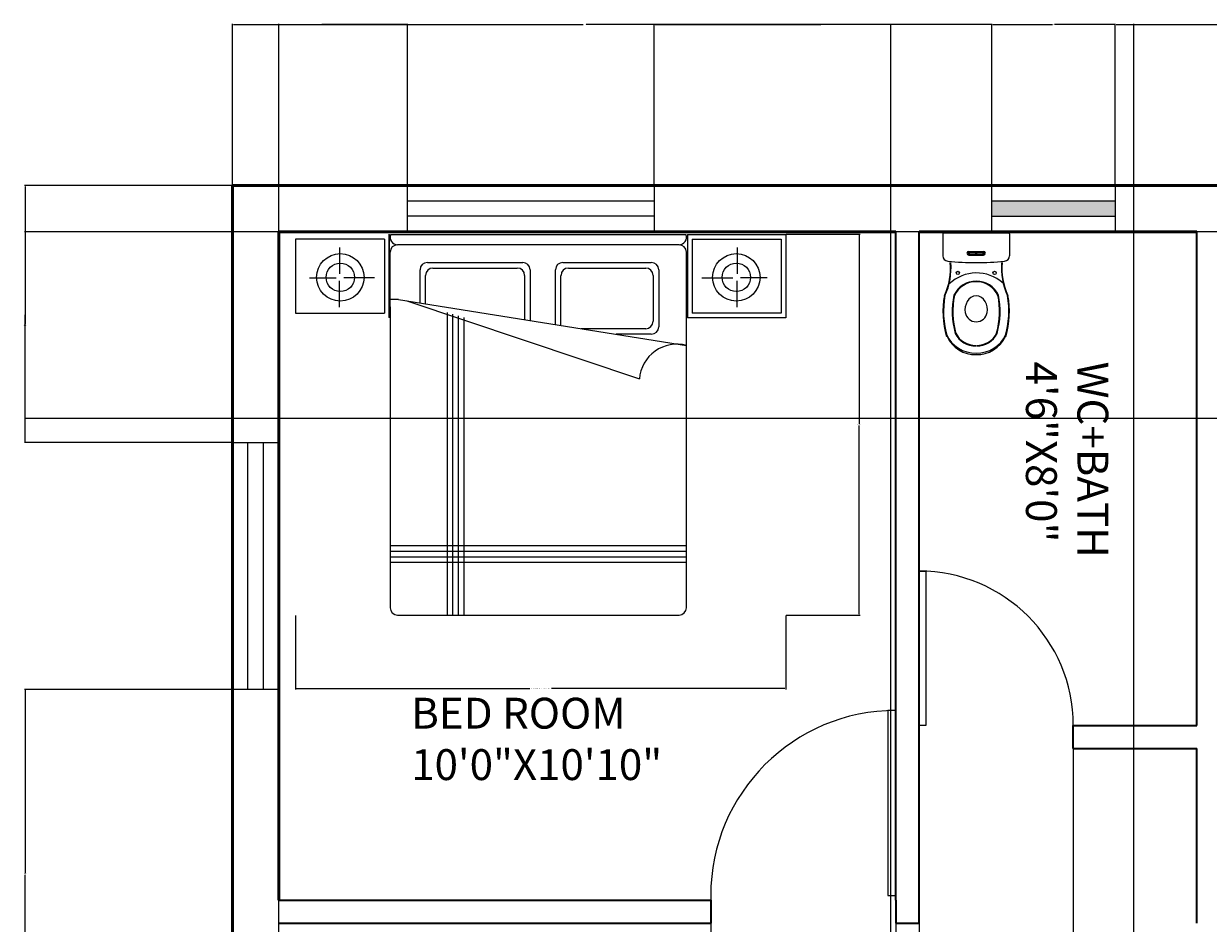
# Model space of a CAD drawing. Units: feet. Extents: x 2664 to 3060, y 1318 to 2005.
# Tile 4 of 5: x 2664 to 2894, y 1830 to 2005. Entities that reach past the tile are written whole.
import ezdxf

# ---------------------------------------------------------------- set-up
doc = ezdxf.new("R2010")
doc.units = ezdxf.units.FT
for name, color, linetype, lineweight in [('A-ANNO-DIMS', 2, 'Continuous', 18), ('A-AREA-IDEN', 109, 'Continuous', 18), ('A-WALL-EXTR', 130, 'Continuous', 50), ('DOOR', 249, 'Continuous', 25), ('FURNITURE', 240, 'Continuous', 13), ('SANITARY', 50, 'Continuous', 13)]:
    doc.layers.add(name, color=color, linetype=linetype, lineweight=lineweight)
for name, color, linetype, lineweight, true_color in [('A-GLAZ', 222, 'Continuous', 18, 0xd4008b), ('A-VENT-PATT', 219, 'Continuous', 13, 0x642165), ('A-WALL-INTR', 41, 'Continuous', 35, 0xf5dd7a), ('VENT', 95, 'Continuous', 18, 0x46b72a)]:
    doc.layers.add(name, color=color, linetype=linetype, lineweight=lineweight, true_color=true_color)
doc.styles.get("Standard").update_dxf_attribs({"font": 'arial.ttf'})
doc.dimstyles.get("Standard").update_dxf_attribs({"dimtxt": 0.18, "dimasz": 0.18, "dimexe": 0.18, "dimexo": 0.0625, "dimgap": 0.09, "dimtad": 0, "dimtih": 1, "dimtoh": 1, "dimdec": 4, "dimzin": 0, "dimdsep": 46, "dimtxsty": 'Standard', "dimcen": 0.09, "dimadec": 0, "dimazin": 0, "dimtfac": 1, "dimtdec": 4, "dimtofl": 0, "dimtmove": 0, "dimatfit": 3, "dimfxl": 1, "dimtolj": 1, "dimtzin": 0, "dimarcsym": 0})

# ---------------------------------------------------------------- blocks, each defined once
blk = doc.blocks.new('*U3')
for p, q in [((0, 0), (0, -6)), ((-40, 0), (-40, -6))]:
    blk.add_line(p, q)
blk.add_lwpolyline([(0, 0), (0, 40), (-1.75, 40), (-1.75, 0)], close=True)
blk.add_arc((0, 0), 40, 90, 180)
blk = doc.blocks.new('*U2')
for p, q in [((0, 0), (0, -6)), ((40, 0), (40, -6))]:
    blk.add_line(p, q)
blk.add_lwpolyline([(0, 0), (0, 40), (1.75, 40), (1.75, 0)], close=True)
blk.add_arc((0, 0), 40, 0, 90)
blk = doc.blocks.new('BED-DOUBLE-WITH-NIGHTSTANDS')
for p, q in [((-29.54, 0), (-29.54, -16.21)), ((-30.37, -0.95), (-47.65, -0.95)), ((-47.65, -0.95), (-47.65, -15.35)), ((-30.37, -0.95), (-30.37, -15.35)), ((-29.47, -0.05), (-29.47, -16.25)), ((28.27, -0.11), (-29.17, -0.11)), ((26.92, -2.06), (-27.82, -2.06)), ((28.57, -0.05), (47.65, -0.05)), ((28.57, -0.05), (28.57, -16.25)), ((29.47, -0.95), (46.75, -0.95)), ((29.47, -0.95), (29.47, -15.35)), ((46.75, -0.95), (46.75, -15.35)), ((47.65, -0.05), (47.65, -16.25)), ((-39.11, -2.58), (-39.11, -7.74)), ((-29.26, -14.16), (-29.26, -3.5)), ((28.36, -72.65), (28.36, -3.5)), ((38.21, -2.58), (38.21, -7.74)), ((-22.01, -5.5), (-3.48, -5.5)), ((-20.93, -6.58), (-4.56, -6.58)), ((4.33, -5.5), (21.52, -5.5)), ((5.41, -6.58), (20.44, -6.58)), ((-44.95, -8.46), (-39.75, -8.46)), ((-39.11, -14.22), (-39.11, -9.06)), ((-32.27, -8.46), (-38.27, -8.46)), ((-23.45, -13.32), (-23.45, -6.94)), ((-22.37, -13.47), (-22.37, -8.02)), ((-3.12, -8.02), (-3.12, -16.63)), ((-2.04, -6.94), (-2.04, -16.8)), ((2.88, -17.58), (2.88, -6.94)), ((3.96, -17.76), (3.96, -8.02)), ((21.88, -8.02), (21.88, -16.94)), ((22.96, -6.94), (22.96, -18.02)), ((31.37, -8.46), (37.37, -8.46)), ((38.21, -14.22), (38.21, -9.06)), ((44.05, -8.46), (38.85, -8.46)), ((-27.62, -12.73), (-29.26, -12.73)), ((-27.62, -12.73), (28.36, -21.64)), ((-26, -12.96), (19.2, -28.15)), ((-47.65, -15.35), (-30.37, -15.35)), ((-29.26, -14.16), (-29.26, -72.65)), ((-18.14, -74.09), (-18.14, -15.24)), ((-17.06, -74.09), (-17.06, -15.55)), ((-15.97, -74.09), (-15.97, -15.86)), ((46.75, -15.35), (29.47, -15.35)), ((-14.89, -74.09), (-14.89, -16.18)), ((20.44, -18.38), (7.87, -18.38)), ((47.65, -16.25), (28.57, -16.25)), ((21.52, -19.46), (14.66, -19.46)), ((28.36, -60.64), (-29.26, -60.64)), ((28.36, -61.72), (-29.26, -61.72)), ((28.36, -62.8), (-29.26, -62.8)), ((28.36, -63.88), (-29.26, -63.88)), ((-27.82, -74.09), (26.92, -74.09))]:
    blk.add_line(p, q)
for centre, radius in [((-38.95, -8.4), 4.61), ((38.05, -8.4), 4.61), ((-38.95, -8.4), 2.77), ((38.05, -8.4), 2.77)]:
    blk.add_circle(centre, radius)
for centre, radius, start, end in [((-27.82, -0.62), 1.44, 159.2884, 270), ((-27.82, -3.5), 1.44, 90, 180), ((26.92, -0.62), 1.44, 270, 20.7116), ((26.92, -3.5), 1.44, 0, 90), ((-22.01, -6.94), 1.44, 90, 180), ((-20.93, -8.02), 1.44, 90, 180), ((-4.56, -8.02), 1.44, 0, 90), ((-3.48, -6.94), 1.44, 0, 90), ((4.33, -6.94), 1.44, 90, 180), ((5.41, -8.02), 1.44, 90, 180), ((20.44, -8.02), 1.44, 0, 90), ((21.52, -6.94), 1.44, 0, 90), ((20.44, -16.94), 1.44, 270, 0), ((21.52, -18.02), 1.44, 270, 0), ((26.5, -28.71), 7.32, 75.237, 175.5647), ((-27.82, -72.65), 1.44, 180, 270), ((26.92, -72.65), 1.44, 270, 0)]:
    blk.add_arc(centre, radius, start, end)
blk = doc.blocks.new('WC-FLOOR-MOUNT')
for p, q in [((-6.3, 0), (6.3, 0)), ((-6.48, -0.18), (-6.48, -4.43)), ((6.48, -0.18), (6.48, -4.43)), ((-1.44, -3.6), (1.44, -3.6)), ((-1.44, -3.71), (1.44, -3.71)), ((-1.44, -3.82), (-0.18, -3.82)), ((-1.44, -4.11), (-0.18, -4.11)), ((-1.44, -4.21), (1.44, -4.21)), ((-1.44, -4.32), (1.44, -4.32)), ((-0.07, -3.93), (-0.07, -4)), ((0.07, -3.93), (0.07, -4)), ((0.18, -3.82), (1.44, -3.82)), ((0.18, -4.11), (1.44, -4.11))]:
    blk.add_line(p, q)
for centre, radius in [((-1.42, -3.96), 0.112), ((-1.42, -3.96), 0.0402), ((1.42, -3.96), 0.112), ((1.42, -3.96), 0.0402), ((-3.57, -7.78), 0.318), ((3.57, -7.78), 0.318)]:
    blk.add_circle(centre, radius)
for centre, radius, start, end in [((-6.3, -0.18), 0.18, 90, 180), ((6.3, -0.18), 0.18, 0, 90), ((-5.4, -4.43), 1.08, 180, 264.6037), ((-1.44, -3.96), 0.36, 90, 180), ((-1.44, -3.96), 0.36, 180, 270), ((-1.44, -3.96), 0.252, 90, 180), ((-1.44, -3.96), 0.252, 180, 270), ((-1.44, -3.96), 0.144, 90, 270), ((-0.18, -3.93), 0.108, 0, 90), ((-0.18, -4), 0.108, 270, 0), ((0.18, -3.93), 0.108, 90, 180), ((0.18, -4), 0.108, 180, 270), ((1.44, -3.96), 0.36, 0, 90), ((1.44, -3.96), 0.252, 0, 90), ((1.44, -3.96), 0.144, 270, 90), ((1.44, -3.96), 0.36, 270, 0), ((1.44, -3.96), 0.252, 270, 0), ((5.4, -4.43), 1.08, 275.3963, 0), ((-17.58, -6.84), 12.59, 334.9634, 4.9109), ((-17.58, -6.84), 12.69, 334.9634, 4.9109), ((0, 52.77), 58.53, 264.6037, 275.3963), ((17.58, -6.84), 12.69, 175.0891, 205.0366), ((17.58, -6.84), 12.59, 175.0891, 205.0366), ((0.06, -15.51), 7.72, 48.0834, 133.5369), ((0, -14.17), 4.8, 25.6263, 154.3737), ((0, -14.17), 4.69, 25.6263, 154.3737), ((11.03, -15.28), 17.49, 169.7326, 196.2187), ((11.03, -15.28), 17.38, 169.7326, 196.2187), ((11.03, -15.28), 15.69, 168.2525, 195.7257), ((11.03, -15.28), 15.58, 168.2525, 196.2187), ((1.08, -14.97), 3.26, 149.7876, 189.0746), ((0, -14.17), 1.92, 25.6263, 154.3737), ((-1.08, -14.97), 3.26, 350.9254, 30.2124), ((-11.03, -15.28), 15.58, 344.3098, 11.7475), ((-11.03, -15.28), 15.69, 344.2743, 11.7475), ((-11.03, -15.28), 17.38, 343.7813, 10.2674), ((-11.03, -15.28), 17.49, 343.7813, 10.2674), ((0, -15.12), 2.16, 189.6495, 350.3505), ((-0.18, -17.24), 6.13, 204.3045, 271.6847), ((-0.18, -17.65), 6.02, 204.3045, 271.6847), ((-0.18, -17.65), 4.32, 205.8912, 271.6847), ((-0.18, -17.65), 4.22, 206.0212, 271.6847), ((0.18, -17.24), 6.13, 268.3153, 335.6955), ((0.18, -17.65), 6.02, 268.3153, 335.6955), ((0.18, -17.65), 4.32, 268.3153, 334.1088), ((0.18, -17.65), 4.22, 268.3153, 333.9788)]:
    blk.add_arc(centre, radius, start, end)
blk = doc.blocks.new('WINDOW-4FT')
for p, q in [((-24, 4.5), (24, 4.5)), ((-24, -4.5), (-24, 4.5)), ((24, 4.5), (24, -4.5)), ((-24, 1.5), (24, 1.5)), ((24, -1.5), (-24, -1.5)), ((24, -4.5), (-24, -4.5))]:
    blk.add_line(p, q)
blk = doc.blocks.new('*D24')
at = {"layer": 'A-ANNO-DIMS', "color": 0, "lineweight": -2, "transparency": 16777216}
for p, q in [((2716.56, 1889.94), (2716.56, 1875.53)), ((2811.86, 1889.94), (2811.86, 1875.53)), ((2716.74, 1875.71), (2762.1, 1875.71)), ((2811.68, 1875.71), (2766.32, 1875.71))]:
    blk.add_line(p, q, dxfattribs=at)
at = {"layer": 'A-ANNO-DIMS', "color": 0, "transparency": 16777216}
for points in [[(2716.74, 1875.74), (2716.74, 1875.68), (2716.56, 1875.71)], [(2811.68, 1875.74), (2811.68, 1875.68), (2811.86, 1875.71)]]:
    blk.add_solid(points, dxfattribs=at)
at = {"layer": 'Defpoints', "color": 0, "transparency": 16777216}
for p in [(2716.56, 1890), (2811.86, 1890), (2811.86, 1875.71)]:
    blk.add_point(p, dxfattribs=at)
at = {"layer": 'A-ANNO-DIMS', "color": 0, "transparency": 16777216, "insert": (2764.21, 1875.71), "char_height": 0.18, "attachment_point": 5}
blk.add_mtext('\\A1;BED WITH NIGHTSTANDS 95 TYP.', dxfattribs=at)
blk = doc.blocks.new('*D25')
at = {"layer": 'A-ANNO-DIMS', "color": 0, "lineweight": -2, "transparency": 16777216}
for p, q in [((2811.92, 1964.1), (2826.33, 1964.1)), ((2826.15, 1963.92), (2826.15, 1927.23)), ((2826.15, 1890.18), (2826.15, 1926.87)), ((2811.92, 1890), (2826.33, 1890))]:
    blk.add_line(p, q, dxfattribs=at)
at = {"layer": 'A-ANNO-DIMS', "color": 0, "transparency": 16777216}
for points in [[(2826.12, 1963.92), (2826.18, 1963.92), (2826.15, 1964.1)], [(2826.12, 1890.18), (2826.18, 1890.18), (2826.15, 1890)]]:
    blk.add_solid(points, dxfattribs=at)
at = {"layer": 'Defpoints', "color": 0, "transparency": 16777216}
for p in [(2811.86, 1964.1), (2826.15, 1964.1), (2811.86, 1890)]:
    blk.add_point(p, dxfattribs=at)
at = {"layer": 'A-ANNO-DIMS', "color": 0, "transparency": 16777216, "insert": (2826.15, 1927.05), "char_height": 0.18, "attachment_point": 5}
blk.add_mtext('\\A1;74 TYP.', dxfattribs=at)
blk = doc.blocks.new('*D35')
at = {"layer": 'A-ANNO-DIMS', "color": 0, "lineweight": -2, "transparency": 16777216}
for p, q in [((2704.28, 1973.63), (2704.28, 2005.03)), ((2704.46, 2004.85), (2720.9, 2004.85)), ((2738.12, 2004.85), (2721.68, 2004.85)), ((2738.3, 1973.63), (2738.3, 2005.03))]:
    blk.add_line(p, q, dxfattribs=at)
at = {"layer": 'A-ANNO-DIMS', "color": 0, "transparency": 16777216}
for points in [[(2704.46, 2004.88), (2704.46, 2004.82), (2704.28, 2004.85)], [(2738.12, 2004.88), (2738.12, 2004.82), (2738.3, 2004.85)]]:
    blk.add_solid(points, dxfattribs=at)
at = {"layer": 'Defpoints', "color": 0, "transparency": 16777216}
for p in [(2738.3, 2004.85), (2704.28, 1973.57), (2738.3, 1973.57)]:
    blk.add_point(p, dxfattribs=at)
at = {"layer": 'A-ANNO-DIMS', "color": 0, "transparency": 16777216, "insert": (2721.29, 2004.85), "char_height": 0.18, "attachment_point": 5}
blk.add_mtext('\\A1;34.02', dxfattribs=at)
blk = doc.blocks.new('*D36')
at = {"layer": 'A-ANNO-DIMS', "color": 0, "lineweight": -2, "transparency": 16777216}
for p, q in [((2786.3, 1973.63), (2786.3, 2005.03)), ((2786.48, 2004.85), (2818.72, 2004.85)), ((2851.75, 2004.85), (2819.51, 2004.85)), ((2851.93, 1973.63), (2851.93, 2005.03))]:
    blk.add_line(p, q, dxfattribs=at)
at = {"layer": 'A-ANNO-DIMS', "color": 0, "transparency": 16777216}
for points in [[(2786.48, 2004.88), (2786.48, 2004.82), (2786.3, 2004.85)], [(2851.75, 2004.88), (2851.75, 2004.82), (2851.93, 2004.85)]]:
    blk.add_solid(points, dxfattribs=at)
at = {"layer": 'Defpoints', "color": 0, "transparency": 16777216}
for p in [(2851.93, 2004.85), (2786.3, 1973.57), (2851.93, 1973.57)]:
    blk.add_point(p, dxfattribs=at)
at = {"layer": 'A-ANNO-DIMS', "color": 0, "transparency": 16777216, "insert": (2819.11, 2004.85), "char_height": 0.18, "attachment_point": 5}
blk.add_mtext('\\A1;65.62', dxfattribs=at)
blk = doc.blocks.new('*D37')
at = {"layer": 'A-ANNO-DIMS', "color": 0, "lineweight": -2, "transparency": 16777216}
for p, q in [((2851.93, 1973.63), (2851.93, 2005.03)), ((2852.11, 2004.85), (2863.71, 2004.85)), ((2875.75, 2004.85), (2864.15, 2004.85)), ((2875.93, 1973.63), (2875.93, 2005.03))]:
    blk.add_line(p, q, dxfattribs=at)
at = {"layer": 'A-ANNO-DIMS', "color": 0, "transparency": 16777216}
for points in [[(2852.11, 2004.88), (2852.11, 2004.82), (2851.93, 2004.85)], [(2875.75, 2004.88), (2875.75, 2004.82), (2875.93, 2004.85)]]:
    blk.add_solid(points, dxfattribs=at)
at = {"layer": 'Defpoints', "color": 0, "transparency": 16777216}
for p in [(2875.93, 2004.85), (2851.93, 1973.57), (2875.93, 1973.57)]:
    blk.add_point(p, dxfattribs=at)
at = {"layer": 'A-ANNO-DIMS', "color": 0, "transparency": 16777216, "insert": (2863.93, 2004.85), "char_height": 0.18, "attachment_point": 5}
blk.add_mtext('\\A1;24', dxfattribs=at)
blk = doc.blocks.new('*D38')
at = {"layer": 'A-ANNO-DIMS', "color": 0, "lineweight": -2, "transparency": 16777216}
for p, q in [((2875.93, 1973.63), (2875.93, 2005.03)), ((2876.11, 2004.85), (2907.35, 2004.85)), ((2939.35, 2004.85), (2908.11, 2004.85)), ((2939.53, 1973.63), (2939.53, 2005.03))]:
    blk.add_line(p, q, dxfattribs=at)
at = {"layer": 'A-ANNO-DIMS', "color": 0, "transparency": 16777216}
for points in [[(2876.11, 2004.88), (2876.11, 2004.82), (2875.93, 2004.85)], [(2939.35, 2004.88), (2939.35, 2004.82), (2939.53, 2004.85)]]:
    blk.add_solid(points, dxfattribs=at)
at = {"layer": 'Defpoints', "color": 0, "transparency": 16777216}
for p in [(2939.53, 2004.85), (2875.93, 1973.57), (2939.53, 1973.57)]:
    blk.add_point(p, dxfattribs=at)
at = {"layer": 'A-ANNO-DIMS', "color": 0, "transparency": 16777216, "insert": (2907.73, 2004.85), "char_height": 0.18, "attachment_point": 5}
blk.add_mtext('\\A1;63.61', dxfattribs=at)
blk = doc.blocks.new('*D40')
at = {"layer": 'A-ANNO-DIMS', "color": 0, "lineweight": -2, "transparency": 16777216}
for p, q in [((2704.22, 1973.57), (2663.82, 1973.57)), ((2664, 1973.39), (2664, 1948.75)), ((2664, 1923.75), (2664, 1948.39)), ((2704.22, 1923.57), (2663.82, 1923.57))]:
    blk.add_line(p, q, dxfattribs=at)
at = {"layer": 'A-ANNO-DIMS', "color": 0, "transparency": 16777216}
for points in [[(2663.97, 1973.39), (2664.03, 1973.39), (2664, 1973.57)], [(2663.97, 1923.75), (2664.03, 1923.75), (2664, 1923.57)]]:
    blk.add_solid(points, dxfattribs=at)
at = {"layer": 'Defpoints', "color": 0, "transparency": 16777216}
for p in [(2704.28, 1973.57), (2664, 1923.57), (2704.28, 1923.57)]:
    blk.add_point(p, dxfattribs=at)
at = {"layer": 'A-ANNO-DIMS', "color": 0, "transparency": 16777216, "insert": (2664, 1948.57), "char_height": 0.18, "attachment_point": 5}
blk.add_mtext('\\A1;50', dxfattribs=at)
blk = doc.blocks.new('*D41')
at = {"layer": 'A-ANNO-DIMS', "color": 0, "lineweight": -2, "transparency": 16777216}
for p, q in [((2704.22, 1875.57), (2663.82, 1875.57)), ((2664, 1875.39), (2664, 1839.85)), ((2664, 1803.95), (2664, 1839.49)), ((2704.22, 1803.77), (2663.82, 1803.77))]:
    blk.add_line(p, q, dxfattribs=at)
at = {"layer": 'A-ANNO-DIMS', "color": 0, "transparency": 16777216}
for points in [[(2663.97, 1875.39), (2664.03, 1875.39), (2664, 1875.57)], [(2663.97, 1803.95), (2664.03, 1803.95), (2664, 1803.77)]]:
    blk.add_solid(points, dxfattribs=at)
at = {"layer": 'Defpoints', "color": 0, "transparency": 16777216}
for p in [(2704.28, 1875.57), (2664, 1803.77), (2704.28, 1803.77)]:
    blk.add_point(p, dxfattribs=at)
at = {"layer": 'A-ANNO-DIMS', "color": 0, "transparency": 16777216, "insert": (2664, 1839.67), "char_height": 0.18, "attachment_point": 5}
blk.add_mtext('\\A1;71.8', dxfattribs=at)
blk = doc.blocks.new('*D47')
at = {"layer": 'A-ANNO-DIMS', "color": 0, "lineweight": -2, "transparency": 16777216}
for p, q in [((3019.22, 1964.57), (2663.82, 1964.57)), ((2664, 1964.39), (2664, 1946.59)), ((2664, 1928.43), (2664, 1946.23)), ((3019.22, 1928.25), (2663.82, 1928.25))]:
    blk.add_line(p, q, dxfattribs=at)
at = {"layer": 'A-ANNO-DIMS', "color": 0, "transparency": 16777216}
for points in [[(2663.97, 1964.39), (2664.03, 1964.39), (2664, 1964.57)], [(2663.97, 1928.43), (2664.03, 1928.43), (2664, 1928.25)]]:
    blk.add_solid(points, dxfattribs=at)
at = {"layer": 'Defpoints', "color": 0, "transparency": 16777216}
for p in [(3019.28, 1964.57), (2664, 1928.25), (3019.28, 1928.25)]:
    blk.add_point(p, dxfattribs=at)
at = {"layer": 'A-ANNO-DIMS', "color": 0, "transparency": 16777216, "insert": (2664, 1946.41), "char_height": 0.18, "attachment_point": 5}
blk.add_mtext('\\A1;36.32', dxfattribs=at)
blk = doc.blocks.new('*D48')
at = {"layer": 'A-ANNO-DIMS', "color": 0, "lineweight": -2, "transparency": 16777216}
for p, q in [((2879.53, 1619.63), (2879.53, 2005.03)), ((2879.71, 2004.85), (2929.25, 2004.85)), ((2979.35, 2004.85), (2929.81, 2004.85)), ((2979.53, 1619.63), (2979.53, 2005.03))]:
    blk.add_line(p, q, dxfattribs=at)
at = {"layer": 'A-ANNO-DIMS', "color": 0, "transparency": 16777216}
for points in [[(2879.71, 2004.88), (2879.71, 2004.82), (2879.53, 2004.85)], [(2979.35, 2004.88), (2979.35, 2004.82), (2979.53, 2004.85)]]:
    blk.add_solid(points, dxfattribs=at)
at = {"layer": 'Defpoints', "color": 0, "transparency": 16777216}
for p in [(2979.53, 2004.85), (2879.53, 1619.57), (2979.53, 1619.57)]:
    blk.add_point(p, dxfattribs=at)
at = {"layer": 'A-ANNO-DIMS', "color": 0, "transparency": 16777216, "insert": (2929.53, 2004.85), "char_height": 0.18, "attachment_point": 5}
blk.add_mtext('\\A1;100', dxfattribs=at)
blk = doc.blocks.new('*D53')
at = {"layer": 'A-ANNO-DIMS', "color": 0, "lineweight": -2, "transparency": 16777216}
for p, q in [((2797.28, 1830.01), (2797.28, 1318.11)), ((2833.28, 1830.01), (2833.28, 1318.11)), ((2797.46, 1318.29), (2815.06, 1318.29)), ((2833.1, 1318.29), (2815.5, 1318.29))]:
    blk.add_line(p, q, dxfattribs=at)
at = {"layer": 'A-ANNO-DIMS', "color": 0, "transparency": 16777216}
for points in [[(2797.46, 1318.32), (2797.46, 1318.26), (2797.28, 1318.29)], [(2833.1, 1318.32), (2833.1, 1318.26), (2833.28, 1318.29)]]:
    blk.add_solid(points, dxfattribs=at)
at = {"layer": 'Defpoints', "color": 0, "transparency": 16777216}
for p in [(2797.28, 1830.07), (2833.28, 1830.07), (2833.28, 1318.29)]:
    blk.add_point(p, dxfattribs=at)
at = {"layer": 'A-ANNO-DIMS', "color": 0, "transparency": 16777216, "insert": (2815.28, 1318.29), "char_height": 0.18, "attachment_point": 5}
blk.add_mtext('\\A1;36', dxfattribs=at)
blk = doc.blocks.new('*D54')
at = {"layer": 'A-ANNO-DIMS', "color": 0, "lineweight": -2, "transparency": 16777216}
for p, q in [((2837.78, 1868.51), (2837.78, 1318.11)), ((2867.78, 1868.51), (2867.78, 1318.11)), ((2837.96, 1318.29), (2852.56, 1318.29)), ((2867.6, 1318.29), (2853, 1318.29))]:
    blk.add_line(p, q, dxfattribs=at)
at = {"layer": 'A-ANNO-DIMS', "color": 0, "transparency": 16777216}
for points in [[(2837.96, 1318.32), (2837.96, 1318.26), (2837.78, 1318.29)], [(2867.6, 1318.32), (2867.6, 1318.26), (2867.78, 1318.29)]]:
    blk.add_solid(points, dxfattribs=at)
at = {"layer": 'Defpoints', "color": 0, "transparency": 16777216}
for p in [(2837.78, 1868.57), (2867.78, 1868.57), (2867.78, 1318.29)]:
    blk.add_point(p, dxfattribs=at)
at = {"layer": 'A-ANNO-DIMS', "color": 0, "transparency": 16777216, "insert": (2852.78, 1318.29), "char_height": 0.18, "attachment_point": 5}
blk.add_mtext('\\A1;30', dxfattribs=at)
blk = doc.blocks.new('*D55')
at = {"layer": 'A-ANNO-DIMS', "color": 0, "lineweight": -2, "transparency": 16777216}
for p, q in [((2833.28, 1830.01), (2833.28, 1318.11)), ((2837.78, 1830.01), (2837.78, 1318.11)), ((2833.46, 1318.29), (2835.27, 1318.29)), ((2837.6, 1318.29), (2835.79, 1318.29))]:
    blk.add_line(p, q, dxfattribs=at)
at = {"layer": 'A-ANNO-DIMS', "color": 0, "transparency": 16777216}
for points in [[(2833.46, 1318.32), (2833.46, 1318.26), (2833.28, 1318.29)], [(2837.6, 1318.32), (2837.6, 1318.26), (2837.78, 1318.29)]]:
    blk.add_solid(points, dxfattribs=at)
at = {"layer": 'Defpoints', "color": 0, "transparency": 16777216}
for p in [(2833.28, 1830.07), (2837.78, 1830.07), (2837.78, 1318.29)]:
    blk.add_point(p, dxfattribs=at)
at = {"layer": 'A-ANNO-DIMS', "color": 0, "transparency": 16777216, "insert": (2835.53, 1318.29), "char_height": 0.18, "attachment_point": 5}
blk.add_mtext('\\A1;4.5', dxfattribs=at)
blk = doc.blocks.new('*D59')
at = {"layer": 'A-ANNO-DIMS', "color": 0, "lineweight": -2, "transparency": 16777216}
for p, q in [((2713.28, 1488.63), (2713.28, 2005.03)), ((2713.46, 2004.85), (2772.5, 2004.85)), ((2832.1, 2004.85), (2773.06, 2004.85)), ((2832.28, 1489.53), (2832.28, 2005.03))]:
    blk.add_line(p, q, dxfattribs=at)
at = {"layer": 'A-ANNO-DIMS', "color": 0, "transparency": 16777216}
for points in [[(2713.46, 2004.88), (2713.46, 2004.82), (2713.28, 2004.85)], [(2832.1, 2004.88), (2832.1, 2004.82), (2832.28, 2004.85)]]:
    blk.add_solid(points, dxfattribs=at)
at = {"layer": 'Defpoints', "color": 0, "transparency": 16777216}
for p in [(2832.28, 2004.85), (2713.28, 1488.57), (2832.28, 1489.47)]:
    blk.add_point(p, dxfattribs=at)
at = {"layer": 'A-ANNO-DIMS', "color": 0, "transparency": 16777216, "insert": (2772.78, 2004.85), "char_height": 0.18, "attachment_point": 5}
blk.add_mtext('\\A1;119', dxfattribs=at)

msp = doc.modelspace()

# ---------------------------------------------------------------- hatches: boundary and pattern name
at = {"layer": 'A-VENT-PATT'}
h = msp.add_hatch(color=256, dxfattribs=at)
h.dxf.hatch_style = 1
h.paths.add_polyline_path([(2875.926, 1967.571), (2875.926, 1970.571), (2851.926, 1970.571), (2851.926, 1967.571)])

# ---------------------------------------------------------------- linework, layer by layer
at = {"layer": 'A-WALL-EXTR'}
for p, q in [((2704.28, 1973.571), (3028.28, 1973.571)), ((2704.28, 1349.571), (2704.28, 1973.571)), ((2713.28, 1964.571), (2833.28, 1964.571)), ((2713.28, 1834.571), (2713.28, 1964.571)), ((2837.78, 1964.571), (2891.78, 1964.571))]:
    msp.add_line(p, q, dxfattribs=at)
at = {"layer": 'A-WALL-INTR'}
for p, q in [((2833.28, 1834.571), (2833.28, 1964.571)), ((2837.78, 1864.071), (2837.78, 1964.571)), ((2891.78, 1868.571), (2891.78, 1964.571)), ((2867.78, 1868.571), (2891.78, 1868.571)), ((2867.78, 1864.071), (2867.78, 1868.571)), ((2837.78, 1830.071), (2837.78, 1864.071)), ((2867.78, 1864.071), (2891.78, 1864.071)), ((2891.78, 1830.071), (2891.78, 1864.071)), ((2713.28, 1834.571), (2797.28, 1834.571)), ((2797.28, 1834.571), (2797.28, 1830.071)), ((2833.28, 1834.571), (2833.28, 1830.071)), ((2713.28, 1830.071), (2797.28, 1830.071)), ((2833.28, 1830.071), (2837.78, 1830.071))]:
    msp.add_line(p, q, dxfattribs=at)
at = {"layer": 'VENT'}
for p, q in [((2851.926, 1973.571), (2875.926, 1973.571)), ((2851.926, 1964.571), (2851.926, 1973.571)), ((2875.926, 1973.571), (2875.926, 1964.571)), ((2851.926, 1970.571), (2875.926, 1970.571)), ((2851.926, 1967.571), (2875.926, 1967.571)), ((2875.926, 1964.571), (2851.926, 1964.571))]:
    msp.add_line(p, q, dxfattribs=at)

# ---------------------------------------------------------------- block references
at = {"layer": 'A-GLAZ'}
msp.add_blockref('WINDOW-4FT', (2762.303, 1969.071), dxfattribs=at)
at = {"layer": 'A-GLAZ', "rotation": 89.99999999999957}
msp.add_blockref('WINDOW-4FT', (2708.78, 1899.571), dxfattribs=at)
at = {"layer": 'DOOR'}
for name, p, xscale, yscale, zscale in [('*U2', (2837.78, 1868.571), 0.7500000000000038, 0.7500000000000038, 0.7500000000000038), ('*U3', (2833.28, 1835.471), 0.899999999999959, 0.899999999999959, 0.899999999999959)]:
    msp.add_blockref(name, p, dxfattribs=dict(at, xscale=xscale, yscale=yscale, zscale=zscale))
at = {"layer": 'FURNITURE'}
msp.add_blockref('BED-DOUBLE-WITH-NIGHTSTANDS', (2764.207, 1964.096), dxfattribs=at)
at = {"layer": 'SANITARY'}
msp.add_blockref('WC-FLOOR-MOUNT', (2848.899, 1964.338), dxfattribs=at)

# ---------------------------------------------------------------- texts
at = {"layer": 'A-AREA-IDEN', "insert": (2874.581, 1939.318), "char_height": 6, "attachment_point": 1, "rotation": 270}
msp.add_mtext_dynamic_manual_height_columns('WC+BATH\\P4\'6"X8\'0"', width=22.955, gutter_width=12.5, heights=[0], dxfattribs=at)
at = {"layer": 'A-AREA-IDEN', "insert": (2739.046, 1873.934), "char_height": 6, "attachment_point": 1}
msp.add_mtext_dynamic_manual_height_columns('BED ROOM \\P10\'0"X10\'10"', width=47.01119, gutter_width=12.5, heights=[0], dxfattribs=at)

# ---------------------------------------------------------------- dimensions: what is measured, and where the dimension line sits
at = {"layer": 'A-ANNO-DIMS'}
for base, p1, p2, override, picture, middle in [((2738.303, 2004.851), (2704.28, 1973.571), (2738.303, 1973.571), {"dimdec": 2, "dimlfac": 1, "dimrnd": 0, "dimzin": 0, "dimdsep": 46, "dimlunit": 2}, '*D35', (2721.292, 2004.851)), ((2832.28, 2004.851), (2713.28, 1488.571), (2832.28, 1489.471), {"dimdec": 0, "dimlfac": 1, "dimrnd": 0, "dimzin": 0, "dimdsep": 46, "dimlunit": 2}, '*D59', (2772.78, 2004.851)), ((2851.926, 2004.851), (2786.303, 1973.571), (2851.926, 1973.571), {"dimdec": 2, "dimlfac": 1, "dimrnd": 0, "dimzin": 0, "dimdsep": 46, "dimlunit": 2}, '*D36', (2819.115, 2004.851)), ((2875.926, 2004.851), (2851.926, 1973.571), (2875.926, 1973.571), {"dimdec": 0, "dimlfac": 1, "dimrnd": 0, "dimzin": 0, "dimdsep": 46, "dimlunit": 2}, '*D37', (2863.926, 2004.851)), ((2939.534, 2004.851), (2875.926, 1973.571), (2939.534, 1973.571), {"dimdec": 2, "dimlfac": 1, "dimrnd": 0, "dimzin": 0, "dimdsep": 46, "dimlunit": 2}, '*D38', (2907.73, 2004.851)), ((2979.53, 2004.851), (2879.53, 1619.571), (2979.53, 1619.571), {"dimdec": 0, "dimlfac": 1, "dimrnd": 0, "dimzin": 0, "dimdsep": 46, "dimlunit": 2}, '*D48', (2929.53, 2004.851)), ((2867.78, 1318.291), (2837.78, 1868.571), (2867.78, 1868.571), {"dimdec": 0, "dimlfac": 1, "dimrnd": 0, "dimzin": 0, "dimdsep": 46, "dimlunit": 2}, '*D54', (2852.78, 1318.291)), ((2833.28, 1318.291), (2797.28, 1830.071), (2833.28, 1830.071), {"dimdec": 0, "dimlfac": 1, "dimrnd": 0, "dimzin": 0, "dimdsep": 46, "dimlunit": 2}, '*D53', (2815.28, 1318.291)), ((2837.78, 1318.291), (2833.28, 1830.071), (2837.78, 1830.071), {"dimdec": 1, "dimlfac": 1, "dimrnd": 0, "dimzin": 0, "dimdsep": 46, "dimlunit": 2}, '*D55', (2835.53, 1318.291))]:
    dim = msp.add_linear_dim(base=base, p1=p1, p2=p2, dimstyle='Standard', override=override, dxfattribs=at)
    dim.commit()
    dim.dimension.update_dxf_attribs({"geometry": picture, "text_midpoint": middle})
for base, p1, p2, override, picture, middle in [((2664, 1923.571), (2704.28, 1973.571), (2704.28, 1923.571), {"dimdec": 0, "dimlfac": 1, "dimrnd": 0, "dimzin": 0, "dimdsep": 46, "dimlunit": 2}, '*D40', (2664, 1948.571)), ((2664, 1928.253), (3019.28, 1964.571), (3019.28, 1928.253), {"dimdec": 2, "dimlfac": 1, "dimrnd": 0, "dimzin": 0, "dimdsep": 46, "dimlunit": 2}, '*D47', (2664, 1946.412)), ((2664, 1803.772), (2704.28, 1875.571), (2704.28, 1803.772), {"dimdec": 1, "dimlfac": 1, "dimrnd": 0, "dimzin": 0, "dimdsep": 46, "dimlunit": 2}, '*D41', (2664, 1839.671))]:
    dim = msp.add_linear_dim(base=base, p1=p1, p2=p2, angle=90, dimstyle='Standard', override=override, dxfattribs=at)
    dim.commit()
    dim.dimension.update_dxf_attribs({"geometry": picture, "text_midpoint": middle})
dim = msp.add_linear_dim(base=(2826.155, 1964.096), p1=(2811.859, 1890.005), p2=(2811.859, 1964.096), angle=90, text='<> TYP.', dimstyle='Standard', override={"dimdec": 0, "dimlfac": 1, "dimrnd": 0, "dimzin": 0, "dimdsep": 46, "dimlunit": 2}, dxfattribs=at)
dim.commit()
dim.dimension.update_dxf_attribs({"geometry": '*D25', "text_midpoint": (2826.155, 1927.05)})
dim = msp.add_linear_dim(base=(2811.859, 1875.709), p1=(2716.555, 1890.005), p2=(2811.859, 1890.005), text='BED WITH NIGHTSTANDS <> TYP.', dimstyle='Standard', override={"dimdec": 0, "dimlfac": 1, "dimrnd": 0, "dimzin": 0, "dimdsep": 46, "dimlunit": 2}, dxfattribs=at)
dim.commit()
dim.dimension.update_dxf_attribs({"geometry": '*D24', "text_midpoint": (2764.207, 1875.709)})

doc.saveas('drawing.dxf')
